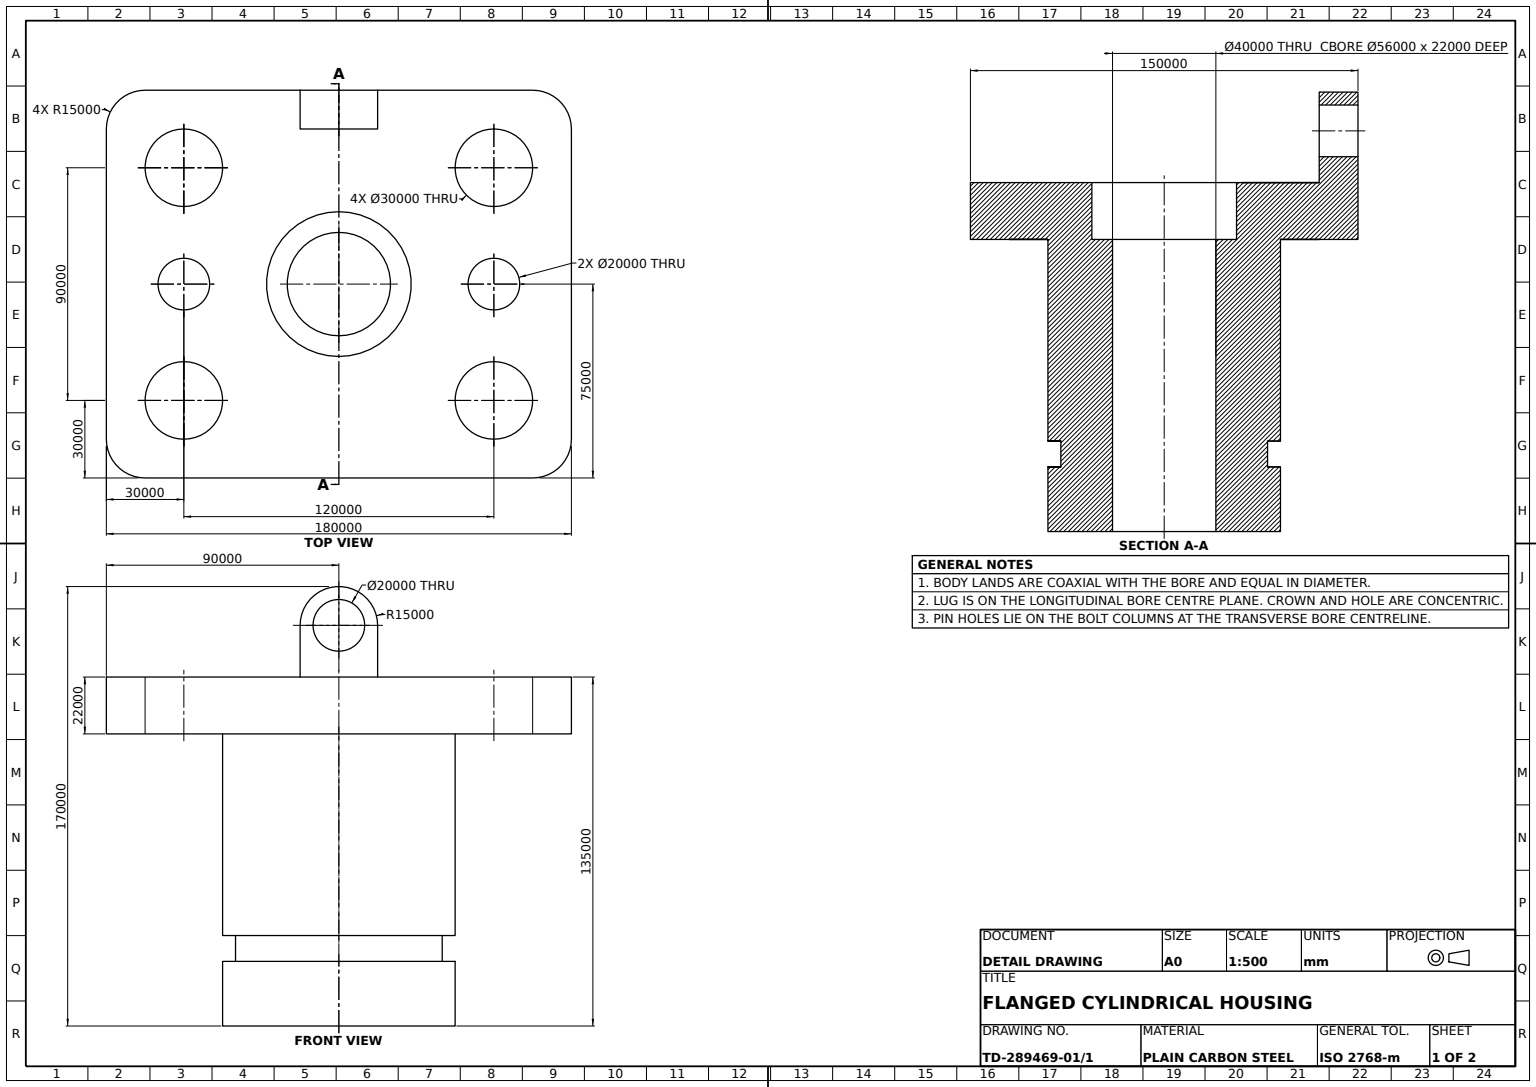
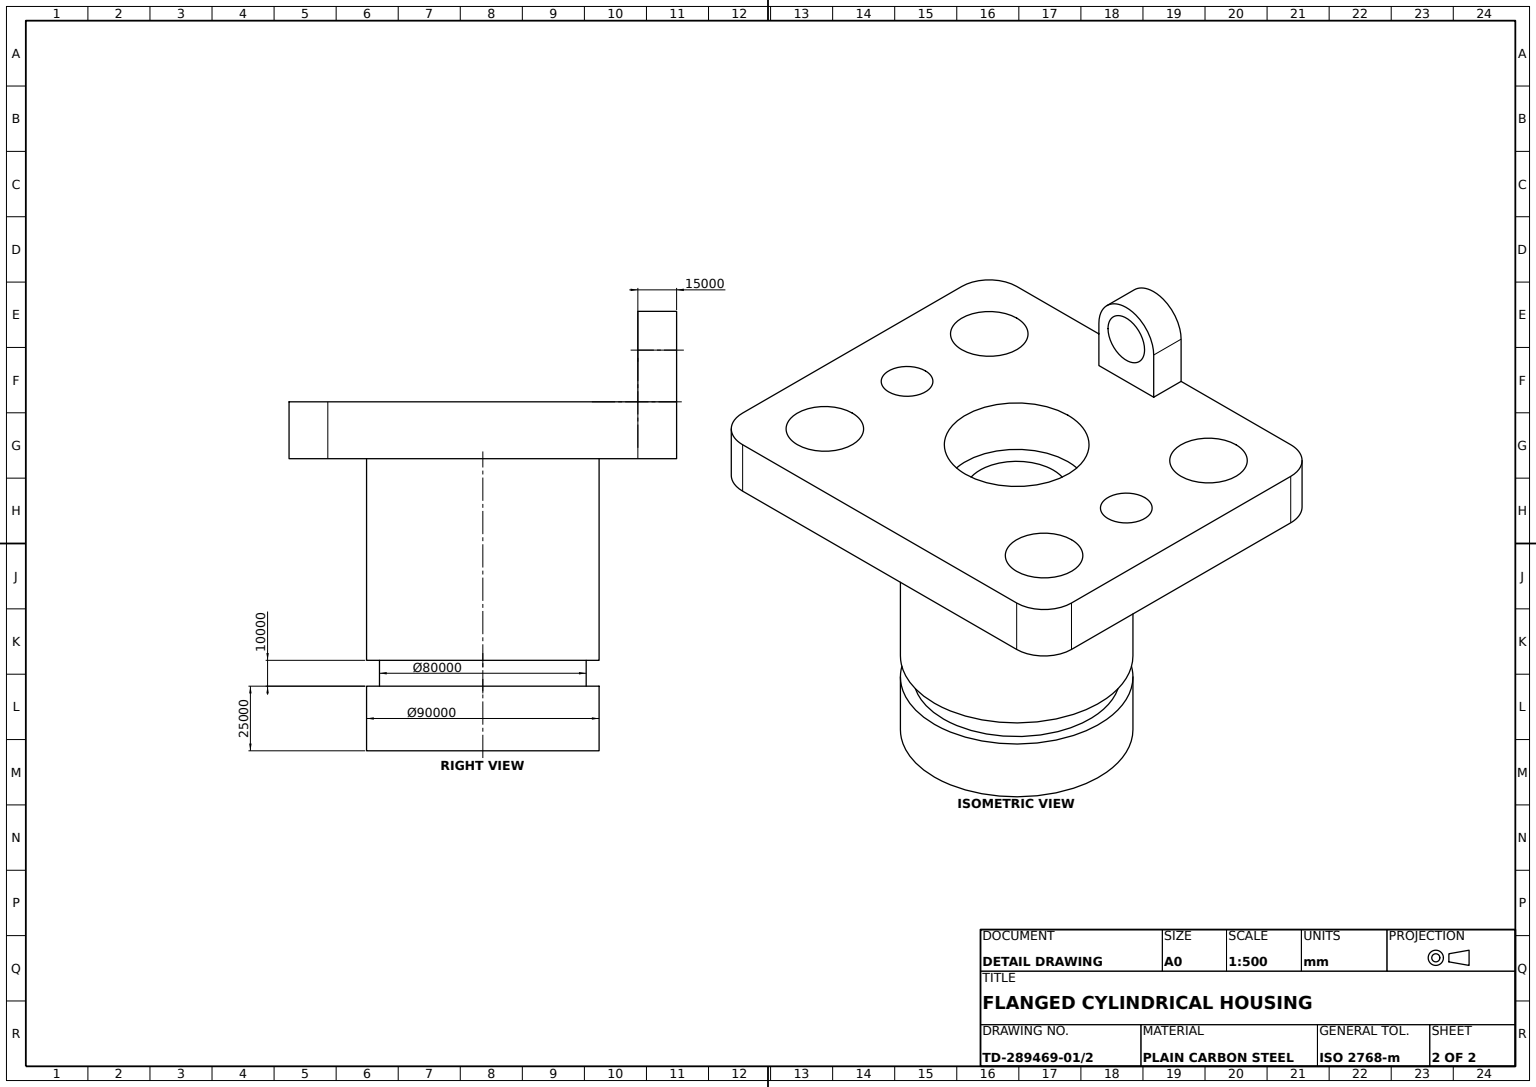
SolidWorks part; units mm, degrees
material "Plain Carbon Steel"
ref_plane "Front Plane" through (0, 0, 0) normal (0, 0, 1) x (1, 0, 0)
ref_plane "Top Plane" through (0, 0, 0) normal (0, 1, 0) x (1, 0, 0)
ref_plane "Right Plane" through (0, 0, 0) normal (1, 0, 0) x (0, 0, -1)
sketch "Plug Body Profile" plane through (0, 0, 0) normal (0, 0, 1) x (1, 0, 0)
  line L1 (-20000, 0) -> (-20000, 121000)
  line L2 (-20000, 121000) -> (-28000, 121000)
  line L3 (-28000, 121000) -> (-28000, 135000)
  line L4 (-28000, 135000) -> (-53000, 135000)
  line L5 (-53000, 135000) -> (-53000, 115000)
  line L6 (-53000, 115000) -> (-45000, 115000)
  line L7 (-45000, 115000) -> (-45000, 35000)
  line L8 (-45000, 35000) -> (-40000, 35000)
  line L9 (-40000, 35000) -> (-40000, 25000)
  line L10 (-40000, 25000) -> (-45000, 25000)
  line L11 (-45000, 25000) -> (-45000, 0)
  line L12 (-45000, 0) -> (-20000, 0)
  line L13 (0, 0) -> (0, 131677.5864) construction
  point P3 (-24000, 121000)
  dimension "D1" = 20000
  dimension "D2" = 121000
  dimension "D3" = 25000
  dimension "D4" = 10000
  dimension "D5" = 28000
  dimension "D6" = 20000
  dimension "D7" = 135000
  dimension "D8" = 5000
  dimension "D9" = 5000
  dimension "D10" = 25000
  dimension "D11" = 25000
  dimension "D12" = 20000
revolve "Plug Body" add sketch "Plug Body Profile" angle 360 about L13
sketch "Flange Profile 180x150" plane through (0, 135000, 0) normal (0, 1, 0) x (1, 0, 0)
  line L1 (-90000, 75000) -> (90000, 75000)
  line L2 (-90000, 75000) -> (-90000, -75000)
  line L3 (-90000, -75000) -> (90000, -75000)
  line L4 (90000, 75000) -> (90000, -75000)
  line L5 (-90000, 75000) -> (90000, -75000) construction
  line L6 (-90000, -75000) -> (90000, 75000) construction
  point P0 (0, 0)
  dimension "D1" = 180000
  dimension "D2" = 150000
extrude "Square Flange" add sketch "Flange Profile 180x150" against normal blind 22000
sketch "Centre Recess Sketch" plane through (0, 135000, 0) normal (0, 1, 0) x (1, 0, 0)
  circle A0 centre (0, 0) radius 28000
  dimension "D1" = 56000
extrude "Centre Recess" cut sketch "Centre Recess Sketch" against normal blind 22000
fillet "Flange Corner Fillet R15 A" radius 15000 1 edges at (90000, 124000, 75000)
fillet "Flange Corner Fillet R15 B" radius 15000 1 edges at (-90000, 124000, 75000)
fillet "Flange Corner Fillet R15 C" radius 15000 1 edges at (-90000, 124000, -75000)
fillet "Flange Corner Fillet R15 D" radius 15000 1 edges at (90000, 124000, -75000)
sketch "Bolt Hole Ø30 A Sketch" plane through (0, 135000, 0) normal (0, 1, 0) x (1, 0, 0)
  line L0 (-75000, -75000) -> (75000, -75000) construction
  line L1 (-90000, 60000) -> (-90000, -60000) construction
  circle A0 centre (-60000, -45000) radius 15000
  dimension "D1" = 30000
  dimension "D2" = 30000
  dimension "D3" = 30000
extrude "Bolt Hole Ø30 A" cut sketch "Bolt Hole Ø30 A Sketch" against normal blind 22000
sketch "Pin Hole Ø20 A Sketch" plane through (0, 135000, 0) normal (0, 1, 0) x (1, 0, 0)
  line L0 (-75000, -75000) -> (75000, -75000) construction
  line L1 (-90000, 60000) -> (-90000, -60000) construction
  circle A0 centre (-60000, 0) radius 10000
  dimension "D1" = 75000
  dimension "D3" = 20000
  dimension "D2" = 30000
extrude "Pin Hole Ø20 A" cut sketch "Pin Hole Ø20 A Sketch" against normal blind 22000
sketch "Bolt Hole Ø30 B Sketch" plane through (0, 135000, 0) normal (0, 1, 0) x (1, 0, 0)
  line L0 (-90000, 60000) -> (-90000, -60000) construction
  line L1 (75000, 75000) -> (-75000, 75000) construction
  circle A0 centre (-60000, 45000) radius 15000
  dimension "D1" = 30000
  dimension "D2" = 30000
  dimension "D3" = 30000
extrude "Bolt Hole Ø30 B" cut sketch "Bolt Hole Ø30 B Sketch" against normal blind 22000
sketch "Bolt Hole Ø30 C Sketch" plane through (0, 135000, 0) normal (0, 1, 0) x (1, 0, 0)
  line L0 (75000, 75000) -> (-75000, 75000) construction
  line L1 (90000, -60000) -> (90000, 60000) construction
  circle A0 centre (60000, 45000) radius 15000
  dimension "D1" = 30000
  dimension "D2" = 30000
  dimension "D3" = 30000
extrude "Bolt Hole Ø30 C" cut sketch "Bolt Hole Ø30 C Sketch" against normal up to next and the other way through all
sketch "Pin Hole Ø20 B Sketch" plane through (0, 135000, 0) normal (0, 1, 0) x (1, 0, 0)
  line L0 (90000, -60000) -> (90000, 60000) construction
  line L1 (75000, 75000) -> (-75000, 75000) construction
  circle A0 centre (60000, 0) radius 10000
  dimension "D1" = 20000
  dimension "D2" = 30000
  dimension "D3" = 75000
extrude "Pin Hole Ø20 B" cut sketch "Pin Hole Ø20 B Sketch" against normal up to next
sketch "Bolt Hole Ø30 D Sketch" plane through (0, 135000, 0) normal (0, 1, 0) x (1, 0, 0)
  line L0 (-75000, -75000) -> (75000, -75000) construction
  line L1 (90000, -60000) -> (90000, 60000) construction
  circle A0 centre (60000, -45000) radius 15000
  dimension "D1" = 30000
  dimension "D2" = 30000
  dimension "D3" = 30000
extrude "Bolt Hole Ø30 D" cut sketch "Bolt Hole Ø30 D Sketch" against normal up to next
sketch "Lifting Lug Profile" plane through (0, 0, -75000) normal (0, 0, -1) x (-1, 0, 0)
  line L0 (0, 135000) -> (15000, 135000)
  line L1 (-75000, 135000) -> (75000, 135000) construction
  line L2 (15000, 135000) -> (15000, 155000)
  line L4 (-15000, 155000) -> (-15000, 135000)
  line L5 (-15000, 135000) -> (0, 135000)
  arc A0 (15000, 155000) -> (-15000, 155000) centre (0, 155000) ccw
  dimension "D4" = 15000
  dimension "D1" = 30000
  dimension "D2" = 15000
  dimension "D3" = 20000
extrude "Lifting Lug" add sketch "Lifting Lug Profile" against normal blind 15000
sketch "Lifting Eye Hole Sketch" plane through (0, 0, -75000) normal (0, 0, -1) x (-1, 0, 0)
  circle A0 centre (0, 155000) radius 10000
  dimension "D1" = 20000
extrude "Lifting Eye Hole" cut sketch "Lifting Eye Hole Sketch" against normal up to next
